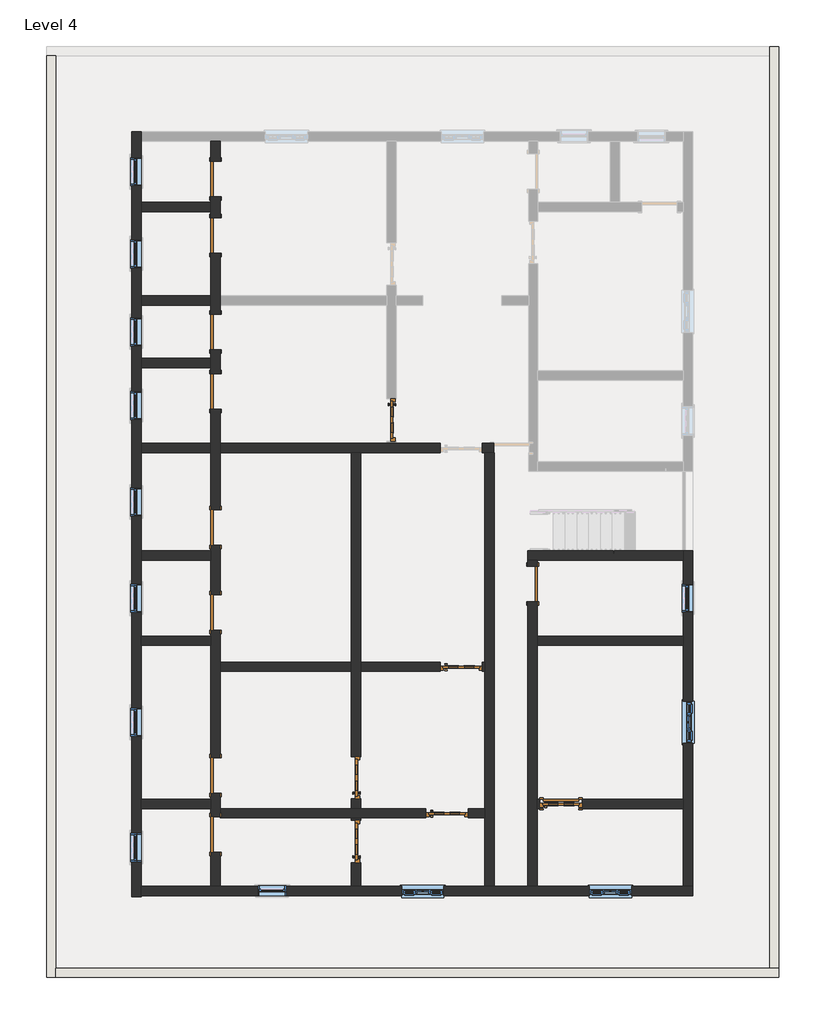
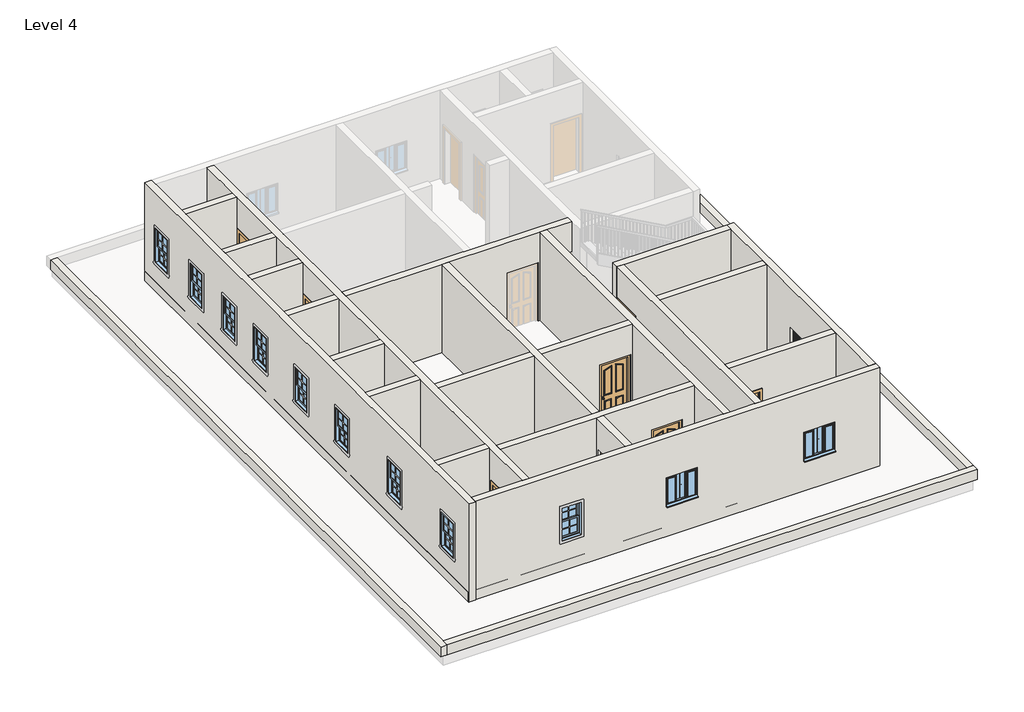
# One storey, part 1 of 3: 22 walls, 16 doors, 13 windows.
"""IFC4 building model written with IfcOpenShell, lengths in millimetres."""

from ifc_helpers import new_model, si_unit, frame, origin, place, context, project, spatial, polyline, outline, extrude, faceted_brep, transform, mapped, element, save
from components import doors_extsgl_12_910x2110mm_9a09825e, doors_extsgl_12_910x2110mm_ece77ece, door_fadea3f2, door_53b1b562, window_679d2811, windows_tpl_w_glazing_cross_bars_910x910mm_4aa0f884

model = new_model("IFC4")

# Units and contexts
model_context = context("Model", 3, world=origin())
ifc_project = project(units=[si_unit("LENGTHUNIT", "METRE", prefix="MILLI")], contexts=[model_context])

# Site, building, storey
site = spatial("IfcSite", under=ifc_project)
building = spatial("IfcBuilding", under=site)
storey = spatial("IfcBuildingStorey", under=building, Name="Level 4", Elevation=9144.0)

# Doors
placement = place(None, origin())
doors_extsgl_12_910x2110mm_shape = doors_extsgl_12_910x2110mm_9a09825e(model_context)
element("IfcDoor", 1, ObjectType="Doors_ExtSgl_12 : 910x2110mm", at=placement, inside=storey, context=model_context, shape_type="MappedRepresentation", body=[
    mapped(doors_extsgl_12_910x2110mm_shape, transform((-4887.6876145, 1213.3404944, 9144.0), x_axis=(0.0, -1.0, 0.0), y_axis=(1.0, 0.0, 0.0), z_axis=(0.0, 0.0, 1.0))),
])
doors_extsgl_12_910x2110mm_2_shape = doors_extsgl_12_910x2110mm_ece77ece(model_context)
element("IfcDoor", 2, ObjectType="Doors_ExtSgl_12 : 910x2110mm", at=placement, inside=storey, context=model_context, shape_type="MappedRepresentation", body=[
    mapped(doors_extsgl_12_910x2110mm_2_shape, transform((-5649.6876145, -6482.8595056, 9144.0), x_axis=(0.0, 1.0, 0.0), y_axis=(-1.0, 0.0, 0.0), z_axis=(0.0, 0.0, 1.0))),
])
element("IfcDoor", 3, ObjectType="Doors_ExtSgl_12 : 910x2110mm", at=placement, inside=storey, context=model_context, shape_type="MappedRepresentation", body=[
    mapped(doors_extsgl_12_910x2110mm_2_shape, transform((-1242.7876145, -7041.6595056, 9144.0), x_axis=(1.0, 0.0, 0.0), y_axis=(0.0, 1.0, 0.0), z_axis=(0.0, 0.0, 1.0))),
])
element("IfcDoor", 4, ObjectType="Doors_ExtSgl_12 : 910x2110mm", at=placement, inside=storey, context=model_context, shape_type="MappedRepresentation", body=[
    mapped(doors_extsgl_12_910x2110mm_2_shape, transform((-5649.6876145, -7854.4595056, 9144.0), x_axis=(0.0, 1.0, 0.0), y_axis=(-1.0, 0.0, 0.0), z_axis=(0.0, 0.0, 1.0))),
])
element("IfcDoor", 5, ObjectType="Doors_ExtSgl_12 : 910x2110mm", at=placement, inside=storey, context=model_context, shape_type="MappedRepresentation", body=[
    mapped(doors_extsgl_12_910x2110mm_2_shape, transform((-3693.8876145, -7244.8595056, 9144.0), x_axis=(1.0, 0.0, 0.0), y_axis=(0.0, 1.0, 0.0), z_axis=(0.0, 0.0, 1.0))),
])
element("IfcDoor", 6, ObjectType="Doors_ExtSgl_12 : 910x2110mm", at=placement, inside=storey, context=model_context, shape_type="MappedRepresentation", body=[
    mapped(doors_extsgl_12_910x2110mm_2_shape, transform((-3389.0876145, -4095.2595056, 9144.0), x_axis=(1.0, 0.0, 0.0), y_axis=(0.0, 1.0, 0.0), z_axis=(0.0, 0.0, 1.0))),
])
door_shape = door_fadea3f2(model_context)
element("IfcDoor", 7, ObjectType="Single-Flush : 30\" x 80\"", at=placement, inside=storey, context=model_context, shape_type="MappedRepresentation", body=[
    mapped(door_shape, transform((-8672.2876145, 5175.7404944, 9144.0), x_axis=(0.0, 1.0, 0.0), y_axis=(-1.0, 0.0, 0.0), z_axis=(0.0, 0.0, 1.0))),
])
element("IfcDoor", 8, ObjectType="Single-Flush : 30\" x 80\"", at=placement, inside=storey, context=model_context, shape_type="MappedRepresentation", body=[
    mapped(door_shape, transform((-8672.2876145, -7702.0595056, 9144.0), x_axis=(0.0, 1.0, 0.0), y_axis=(-1.0, 0.0, 0.0), z_axis=(0.0, 0.0, 1.0))),
])
element("IfcDoor", 9, ObjectType="Single-Flush : 30\" x 80\"", at=placement, inside=storey, context=model_context, shape_type="MappedRepresentation", body=[
    mapped(door_shape, transform((-1852.3876145, -2317.2595056, 9144.0), x_axis=(0.0, -1.0, 0.0), y_axis=(1.0, 0.0, 0.0), z_axis=(0.0, 0.0, 1.0))),
])
element("IfcDoor", 10, ObjectType="Single-Flush : 30\" x 80\"", at=placement, inside=storey, context=model_context, shape_type="MappedRepresentation", body=[
    mapped(door_shape, transform((-1242.7876145, -7041.6595056, 9144.0), x_axis=(1.0, 0.0, 0.0), y_axis=(0.0, 1.0, 0.0), z_axis=(0.0, 0.0, 1.0))),
])
door_2_shape = door_53b1b562(model_context)
element("IfcDoor", 11, ObjectType="Single-Flush : 30\" x 80\"", at=placement, inside=storey, context=model_context, shape_type="MappedRepresentation", body=[
    mapped(door_2_shape, transform((-8672.2876145, 6394.9404944, 9144.0), x_axis=(0.0, -1.0, 0.0), y_axis=(1.0, 0.0, 0.0), z_axis=(0.0, 0.0, 1.0))),
])
element("IfcDoor", 12, ObjectType="Single-Flush : 30\" x 80\"", at=placement, inside=storey, context=model_context, shape_type="MappedRepresentation", body=[
    mapped(door_2_shape, transform((-8672.2876145, 3105.6404944, 9144.0), x_axis=(0.0, -1.0, 0.0), y_axis=(1.0, 0.0, 0.0), z_axis=(0.0, 0.0, 1.0))),
])
element("IfcDoor", 13, ObjectType="Single-Flush : 30\" x 80\"", at=placement, inside=storey, context=model_context, shape_type="MappedRepresentation", body=[
    mapped(door_2_shape, transform((-8672.2876145, 1822.9404944, 9144.0), x_axis=(0.0, -1.0, 0.0), y_axis=(1.0, 0.0, 0.0), z_axis=(0.0, 0.0, 1.0))),
])
element("IfcDoor", 14, ObjectType="Single-Flush : 30\" x 80\"", at=placement, inside=storey, context=model_context, shape_type="MappedRepresentation", body=[
    mapped(door_2_shape, transform((-8672.2876145, -1098.0595056, 9144.0), x_axis=(0.0, -1.0, 0.0), y_axis=(1.0, 0.0, 0.0), z_axis=(0.0, 0.0, 1.0))),
])
element("IfcDoor", 15, ObjectType="Single-Flush : 30\" x 80\"", at=placement, inside=storey, context=model_context, shape_type="MappedRepresentation", body=[
    mapped(door_2_shape, transform((-8672.2876145, -2926.8595056, 9144.0), x_axis=(0.0, -1.0, 0.0), y_axis=(1.0, 0.0, 0.0), z_axis=(0.0, 0.0, 1.0))),
])
element("IfcDoor", 16, ObjectType="Single-Flush : 30\" x 80\"", at=placement, inside=storey, context=model_context, shape_type="MappedRepresentation", body=[
    mapped(door_2_shape, transform((-8672.2876145, -6432.0595056, 9144.0), x_axis=(0.0, -1.0, 0.0), y_axis=(1.0, 0.0, 0.0), z_axis=(0.0, 0.0, 1.0))),
])

# Walls
element("IfcWall", 17, ObjectType="4.5\"", at=placement, inside=storey, context=model_context, shape_type="Brep", body=[
    faceted_brep([(-8773.8876145, -6813.0595056, 9144.0), (-8773.8876145, -6940.0595056, 9144.0), (-8773.8876145, -7143.2595056, 9144.0), (-8773.8876145, -7321.0595056, 9144.0), (-8773.8876145, -7321.0595056, 11176.0), (-8773.8876145, -8083.0595056, 11176.0), (-8773.8876145, -8083.0595056, 9144.0), (-8773.8876145, -8819.6595056, 9144.0), (-8773.8876145, -8819.6595056, 12192.0), (-8773.8876145, -7143.2595056, 12192.0), (-8773.8876145, -6940.0595056, 12192.0), (-8773.8876145, -3638.0595056, 12192.0), (-8773.8876145, -3434.8595056, 12192.0), (-8773.8876145, -1809.2595056, 12192.0), (-8773.8876145, -1606.0595056, 12192.0), (-8773.8876145, 502.1404944, 12192.0), (-8773.8876145, 705.3404944, 12192.0), (-8773.8876145, 2330.9404944, 12192.0), (-8773.8876145, 2534.1404944, 12192.0), (-8773.8876145, 3677.1404944, 12192.0), (-8773.8876145, 3880.3404944, 12192.0), (-8773.8876145, 5683.7404944, 12192.0), (-8773.8876145, 5886.9404944, 12192.0), (-8773.8876145, 7207.7404944, 12192.0), (-8773.8876145, 7207.7404944, 9144.0), (-8773.8876145, 6775.9404944, 9144.0), (-8773.8876145, 6775.9404944, 11176.0), (-8773.8876145, 6013.9404944, 11176.0), (-8773.8876145, 6013.9404944, 9144.0), (-8773.8876145, 5886.9404944, 9144.0), (-8773.8876145, 5683.7404944, 9144.0), (-8773.8876145, 5556.7404944, 9144.0), (-8773.8876145, 5556.7404944, 11176.0), (-8773.8876145, 4794.7404944, 11176.0), (-8773.8876145, 4794.7404944, 9144.0), (-8773.8876145, 3880.3404944, 9144.0), (-8773.8876145, 3677.1404944, 9144.0), (-8773.8876145, 3486.6404944, 9144.0), (-8773.8876145, 3486.6404944, 11176.0), (-8773.8876145, 2724.6404944, 11176.0), (-8773.8876145, 2724.6404944, 9144.0), (-8773.8876145, 2534.1404944, 9144.0), (-8773.8876145, 2330.9404944, 9144.0), (-8773.8876145, 2203.9404944, 9144.0), (-8773.8876145, 2203.9404944, 11176.0), (-8773.8876145, 1441.9404944, 11176.0), (-8773.8876145, 1441.9404944, 9144.0), (-8773.8876145, 705.3404944, 9144.0), (-8773.8876145, 502.1404944, 9144.0), (-8773.8876145, -717.0595056, 9144.0), (-8773.8876145, -717.0595056, 11176.0), (-8773.8876145, -1479.0595056, 11176.0), (-8773.8876145, -1479.0595056, 9144.0), (-8773.8876145, -1606.0595056, 9144.0), (-8773.8876145, -1809.2595056, 9144.0), (-8773.8876145, -2545.8595056, 9144.0), (-8773.8876145, -2545.8595056, 11176.0), (-8773.8876145, -3307.8595056, 11176.0), (-8773.8876145, -3307.8595056, 9144.0), (-8773.8876145, -3434.8595056, 9144.0), (-8773.8876145, -3638.0595056, 9144.0), (-8773.8876145, -6051.0595056, 9144.0), (-8773.8876145, -6051.0595056, 11176.0), (-8773.8876145, -6813.0595056, 11176.0), (-8570.6876145, -7321.0595056, 11176.0), (-8570.6876145, -7321.0595056, 9144.0), (-8570.6876145, -7143.2595056, 9144.0), (-8570.6876145, -6813.0595056, 9144.0), (-8570.6876145, -6813.0595056, 11176.0), (-8570.6876145, -6051.0595056, 11176.0), (-8570.6876145, -6051.0595056, 9144.0), (-8570.6876145, -4196.8595056, 9144.0), (-8570.6876145, -3993.6595056, 9144.0), (-8570.6876145, -3307.8595056, 9144.0), (-8570.6876145, -3307.8595056, 11176.0), (-8570.6876145, -2545.8595056, 11176.0), (-8570.6876145, -2545.8595056, 9144.0), (-8570.6876145, -1479.0595056, 9144.0), (-8570.6876145, -1479.0595056, 11176.0), (-8570.6876145, -717.0595056, 11176.0), (-8570.6876145, -717.0595056, 9144.0), (-8570.6876145, 502.1404944, 9144.0), (-8570.6876145, 705.3404944, 9144.0), (-8570.6876145, 1441.9404944, 9144.0), (-8570.6876145, 1441.9404944, 11176.0), (-8570.6876145, 2203.9404944, 11176.0), (-8570.6876145, 2203.9404944, 9144.0), (-8570.6876145, 2724.6404944, 9144.0), (-8570.6876145, 2724.6404944, 11176.0), (-8570.6876145, 3486.6404944, 11176.0), (-8570.6876145, 3486.6404944, 9144.0), (-8570.6876145, 3677.1404944, 9144.0), (-8570.6876145, 3880.3404944, 9144.0), (-8570.6876145, 4794.7404944, 9144.0), (-8570.6876145, 4794.7404944, 11176.0), (-8570.6876145, 5556.7404944, 11176.0), (-8570.6876145, 5556.7404944, 9144.0), (-8570.6876145, 6013.9404944, 9144.0), (-8570.6876145, 6013.9404944, 11176.0), (-8570.6876145, 6775.9404944, 11176.0), (-8570.6876145, 6775.9404944, 9144.0), (-8570.6876145, 7207.7404944, 9144.0), (-8570.6876145, 7207.7404944, 12192.0), (-8570.6876145, 3880.3404944, 12192.0), (-8570.6876145, 3677.1404944, 12192.0), (-8570.6876145, 705.3404944, 12192.0), (-8570.6876145, 502.1404944, 12192.0), (-8570.6876145, -3993.6595056, 12192.0), (-8570.6876145, -4196.8595056, 12192.0), (-8570.6876145, -7143.2595056, 12192.0), (-8570.6876145, -7346.4595056, 12192.0), (-8570.6876145, -8819.6595056, 12192.0), (-8570.6876145, -8819.6595056, 9144.0), (-8570.6876145, -8083.0595056, 9144.0), (-8570.6876145, -8083.0595056, 11176.0)], [[[0, 1, 2, 3, 4, 5, 6, 7, 8, 9, 10, 11, 12, 13, 14, 15, 16, 17, 18, 19, 20, 21, 22, 23, 24, 25, 26, 27, 28, 29, 30, 31, 32, 33, 34, 35, 36, 37, 38, 39, 40, 41, 42, 43, 44, 45, 46, 47, 48, 49, 50, 51, 52, 53, 54, 55, 56, 57, 58, 59, 60, 61, 62, 63]], [[64, 65, 66, 67, 68, 69, 70, 71, 72, 73, 74, 75, 76, 77, 78, 79, 80, 81, 82, 83, 84, 85, 86, 87, 88, 89, 90, 91, 92, 93, 94, 95, 96, 97, 98, 99, 100, 101, 102, 103, 104, 105, 106, 107, 108, 109, 110, 111, 112, 113, 114]], [[25, 24, 101, 100]], [[97, 96, 31, 30, 29, 28]], [[37, 36, 35, 34, 93, 92, 91, 90]], [[43, 42, 41, 40, 87, 86]], [[49, 48, 47, 46, 83, 82, 81, 80]], [[55, 54, 53, 52, 77, 76]], [[61, 60, 59, 58, 73, 72, 71, 70]], [[113, 112, 7, 6]], [[67, 66, 65, 3, 2, 1, 0]], [[23, 22, 21, 20, 19, 18, 17, 16, 15, 14, 13, 12, 11, 10, 9, 8, 111, 110, 109, 108, 107, 106, 105, 104, 103, 102]], [[8, 7, 112, 111]], [[24, 23, 102, 101]], [[98, 97, 28, 27]], [[99, 98, 27, 26]], [[100, 99, 26, 25]], [[32, 31, 96, 95]], [[33, 32, 95, 94]], [[34, 33, 94, 93]], [[88, 87, 40, 39]], [[89, 88, 39, 38]], [[90, 89, 38, 37]], [[84, 83, 46, 45]], [[85, 84, 45, 44]], [[86, 85, 44, 43]], [[78, 77, 52, 51]], [[79, 78, 51, 50]], [[80, 79, 50, 49]], [[74, 73, 58, 57]], [[75, 74, 57, 56]], [[76, 75, 56, 55]], [[68, 67, 0, 63]], [[69, 68, 63, 62]], [[70, 69, 62, 61]], [[4, 3, 65, 64]], [[5, 4, 64, 114]], [[6, 5, 114, 113]]]),
])
element("IfcWall", 18, ObjectType="4.5\"", at=placement, inside=storey, context=model_context, shape_type="SweptSolid", body=[
    extrude(outline(polyline([(-8773.8876145, 5683.7404944), (-10272.4876145, 5683.7404944), (-10272.4876145, 5886.9404944), (-8773.8876145, 5886.9404944), (-8773.8876145, 5683.7404944)])), frame((0.0, 0.0, 9144.0), z_axis=(0.0, 0.0, 1.0), x_axis=(1.0, 0.0, 0.0)), (0.0, 0.0, 1.0), 3048.0),
])
element("IfcWall", 19, ObjectType="4.5\"", at=placement, inside=storey, context=model_context, shape_type="SweptSolid", body=[
    extrude(outline(polyline([(-8773.8876145, 3677.1404944), (-10272.4876145, 3677.1404944), (-10272.4876145, 3880.3404944), (-8773.8876145, 3880.3404944), (-8773.8876145, 3677.1404944)])), frame((0.0, 0.0, 9144.0), z_axis=(0.0, 0.0, 1.0), x_axis=(1.0, 0.0, 0.0)), (0.0, 0.0, 1.0), 3048.0),
])
element("IfcWall", 20, ObjectType="4.5\"", at=placement, inside=storey, context=model_context, shape_type="SweptSolid", body=[
    extrude(outline(polyline([(-8773.8876145, 2330.9404944), (-10272.4876145, 2330.9404944), (-10272.4876145, 2534.1404944), (-8773.8876145, 2534.1404944), (-8773.8876145, 2330.9404944)])), frame((0.0, 0.0, 9144.0), z_axis=(0.0, 0.0, 1.0), x_axis=(1.0, 0.0, 0.0)), (0.0, 0.0, 1.0), 3048.0),
])
element("IfcWall", 21, ObjectType="4.5\"", at=placement, inside=storey, context=model_context, shape_type="Brep", body=[
    faceted_brep([(-10272.4876145, 502.1404944, 12192.0), (-10272.4876145, 502.1404944, 9144.0), (-8773.8876145, 502.1404944, 9144.0), (-8773.8876145, 502.1404944, 12192.0), (-10272.4876145, 705.3404944, 9144.0), (-10272.4876145, 705.3404944, 12192.0), (-8773.8876145, 705.3404944, 12192.0), (-8773.8876145, 705.3404944, 9144.0)], [[[0, 1, 2, 3]], [[4, 5, 6, 7]], [[1, 4, 7, 2]], [[5, 0, 3, 6]], [[1, 0, 5, 4]], [[3, 2, 7, 6]]]),
    faceted_brep([(-1941.2876145, 502.1404944, 11176.0), (-1941.2876145, 502.1404944, 12192.0), (-2677.8876145, 502.1404944, 12192.0), (-2881.0876145, 502.1404944, 12192.0), (-5548.0876145, 502.1404944, 12192.0), (-5751.2876145, 502.1404944, 12192.0), (-8570.6876145, 502.1404944, 12192.0), (-8570.6876145, 502.1404944, 9144.0), (-5751.2876145, 502.1404944, 9144.0), (-5548.0876145, 502.1404944, 9144.0), (-3844.0876145, 502.1404944, 9144.0), (-3844.0876145, 502.1404944, 11254.0), (-2934.0876145, 502.1404944, 11254.0), (-2934.0876145, 502.1404944, 9144.0), (-2881.0876145, 502.1404944, 9144.0), (-2690.5876145, 502.1404944, 9144.0), (-2690.5876145, 502.1404944, 11176.0), (-1941.2876145, 705.3404944, 12192.0), (-1941.2876145, 705.3404944, 11176.0), (-2690.5876145, 705.3404944, 11176.0), (-2690.5876145, 705.3404944, 9144.0), (-2934.0876145, 705.3404944, 9144.0), (-2934.0876145, 705.3404944, 11254.0), (-3844.0876145, 705.3404944, 11254.0), (-3844.0876145, 705.3404944, 9144.0), (-4786.0876145, 705.3404944, 9144.0), (-4989.2876145, 705.3404944, 9144.0), (-8570.6876145, 705.3404944, 9144.0), (-8570.6876145, 705.3404944, 12192.0), (-4989.2876145, 705.3404944, 12192.0), (-4786.0876145, 705.3404944, 12192.0)], [[[0, 1, 2, 3, 4, 5, 6, 7, 8, 9, 10, 11, 12, 13, 14, 15, 16]], [[17, 18, 19, 20, 21, 22, 23, 24, 25, 26, 27, 28, 29, 30]], [[20, 15, 14, 13, 21]], [[24, 10, 9, 8, 7, 27, 26, 25]], [[1, 17, 30, 29, 28, 6, 5, 4, 3, 2]], [[7, 6, 28, 27]], [[17, 1, 0, 18]], [[16, 19, 18, 0]], [[19, 16, 15, 20]], [[24, 23, 11, 10]], [[22, 21, 13, 12]], [[23, 22, 12, 11]]]),
])
element("IfcWall", 22, ObjectType="4.5\"", at=placement, inside=storey, context=model_context, shape_type="SweptSolid", body=[
    extrude(outline(polyline([(-8773.8876145, -1809.2595056), (-10272.4876145, -1809.2595056), (-10272.4876145, -1606.0595056), (-8773.8876145, -1606.0595056), (-8773.8876145, -1809.2595056)])), frame((0.0, 0.0, 9144.0), z_axis=(0.0, 0.0, 1.0), x_axis=(1.0, 0.0, 0.0)), (0.0, 0.0, 1.0), 3048.0),
])
element("IfcWall", 23, ObjectType="4.5\"", at=placement, inside=storey, context=model_context, shape_type="SweptSolid", body=[
    extrude(outline(polyline([(-8773.8876145, -3638.0595056), (-10272.4876145, -3638.0595056), (-10272.4876145, -3434.8595056), (-8773.8876145, -3434.8595056), (-8773.8876145, -3638.0595056)])), frame((0.0, 0.0, 9144.0), z_axis=(0.0, 0.0, 1.0), x_axis=(1.0, 0.0, 0.0)), (0.0, 0.0, 1.0), 3048.0),
])
element("IfcWall", 24, ObjectType="4.5\"", at=placement, inside=storey, context=model_context, shape_type="SweptSolid", body=[
    extrude(outline(polyline([(-8773.8876145, -7143.2595056), (-10272.4876145, -7143.2595056), (-10272.4876145, -6940.0595056), (-8773.8876145, -6940.0595056), (-8773.8876145, -7143.2595056)])), frame((0.0, 0.0, 9144.0), z_axis=(0.0, 0.0, 1.0), x_axis=(1.0, 0.0, 0.0)), (0.0, 0.0, 1.0), 3048.0),
])
element("IfcWall", 25, ObjectType="4.5\"", at=placement, inside=storey, context=model_context, shape_type="Brep", body=[
    faceted_brep([(-3238.8876145, -7346.4595056, 11254.0), (-3238.8876145, -7346.4595056, 9144.0), (-2881.0876145, -7346.4595056, 9144.0), (-2881.0876145, -7346.4595056, 12192.0), (-5548.0876145, -7346.4595056, 12192.0), (-5751.2876145, -7346.4595056, 12192.0), (-8570.6876145, -7346.4595056, 12192.0), (-8570.6876145, -7346.4595056, 9144.0), (-5751.2876145, -7346.4595056, 9144.0), (-5548.0876145, -7346.4595056, 9144.0), (-4148.8876145, -7346.4595056, 9144.0), (-4148.8876145, -7346.4595056, 11254.0), (-2881.0876145, -7143.2595056, 9144.0), (-3238.8876145, -7143.2595056, 9144.0), (-3238.8876145, -7143.2595056, 11254.0), (-4148.8876145, -7143.2595056, 11254.0), (-4148.8876145, -7143.2595056, 9144.0), (-5548.0876145, -7143.2595056, 9144.0), (-5751.2876145, -7143.2595056, 9144.0), (-8570.6876145, -7143.2595056, 9144.0), (-8570.6876145, -7143.2595056, 12192.0), (-5751.2876145, -7143.2595056, 12192.0), (-5548.0876145, -7143.2595056, 12192.0), (-2881.0876145, -7143.2595056, 12192.0), (-8570.6876145, -7321.0595056, 9144.0)], [[[0, 1, 2, 3, 4, 5, 6, 7, 8, 9, 10, 11]], [[12, 13, 14, 15, 16, 17, 18, 19, 20, 21, 22, 23]], [[2, 1, 13, 12]], [[10, 9, 8, 7, 24, 19, 18, 17, 16]], [[6, 5, 4, 3, 23, 22, 21, 20]], [[7, 6, 20, 19, 24]], [[3, 2, 12, 23]], [[16, 15, 11, 10]], [[14, 13, 1, 0]], [[15, 14, 0, 11]]]),
])
element("IfcWall", 26, ObjectType="4.5\"", at=placement, inside=storey, context=model_context, shape_type="Brep", body=[
    faceted_brep([(-5751.2876145, -8819.6595056, 9144.0), (-5751.2876145, -8819.6595056, 12192.0), (-5751.2876145, -7346.4595056, 12192.0), (-5751.2876145, -7346.4595056, 9144.0), (-5751.2876145, -7399.4595056, 9144.0), (-5751.2876145, -7399.4595056, 11254.0), (-5751.2876145, -8309.4595056, 11254.0), (-5751.2876145, -8309.4595056, 9144.0), (-5548.0876145, -8819.6595056, 12192.0), (-5548.0876145, -8819.6595056, 9144.0), (-5548.0876145, -8309.4595056, 9144.0), (-5548.0876145, -8309.4595056, 11254.0), (-5548.0876145, -7399.4595056, 11254.0), (-5548.0876145, -7399.4595056, 9144.0), (-5548.0876145, -7346.4595056, 9144.0), (-5548.0876145, -7346.4595056, 12192.0)], [[[0, 1, 2, 3, 4, 5, 6, 7]], [[8, 9, 10, 11, 12, 13, 14, 15]], [[9, 0, 7, 10]], [[13, 4, 3, 14]], [[1, 8, 15, 2]], [[1, 0, 9, 8]], [[3, 2, 15, 14]], [[7, 6, 11, 10]], [[5, 4, 13, 12]], [[6, 5, 12, 11]]]),
    faceted_brep([(-5751.2876145, 502.1404944, 12192.0), (-5751.2876145, 502.1404944, 9144.0), (-5751.2876145, -3993.6595056, 9144.0), (-5751.2876145, -4196.8595056, 9144.0), (-5751.2876145, -6027.8595056, 9144.0), (-5751.2876145, -6027.8595056, 11254.0), (-5751.2876145, -6937.8595056, 11254.0), (-5751.2876145, -6937.8595056, 9144.0), (-5751.2876145, -7143.2595056, 9144.0), (-5751.2876145, -7143.2595056, 12192.0), (-5751.2876145, -4196.8595056, 12192.0), (-5751.2876145, -3993.6595056, 12192.0), (-5548.0876145, 502.1404944, 9144.0), (-5548.0876145, 502.1404944, 12192.0), (-5548.0876145, -3993.6595056, 12192.0), (-5548.0876145, -4196.8595056, 12192.0), (-5548.0876145, -7143.2595056, 12192.0), (-5548.0876145, -7143.2595056, 9144.0), (-5548.0876145, -6937.8595056, 9144.0), (-5548.0876145, -6937.8595056, 11254.0), (-5548.0876145, -6027.8595056, 11254.0), (-5548.0876145, -6027.8595056, 9144.0), (-5548.0876145, -4196.8595056, 9144.0), (-5548.0876145, -3993.6595056, 9144.0)], [[[0, 1, 2, 3, 4, 5, 6, 7, 8, 9, 10, 11]], [[12, 13, 14, 15, 16, 17, 18, 19, 20, 21, 22, 23]], [[1, 12, 23, 22, 21, 4, 3, 2]], [[7, 18, 17, 8]], [[13, 0, 11, 10, 9, 16, 15, 14]], [[1, 0, 13, 12]], [[9, 8, 17, 16]], [[7, 6, 19, 18]], [[5, 4, 21, 20]], [[6, 5, 20, 19]]]),
])
element("IfcWall", 27, ObjectType="4.5\"", at=placement, inside=storey, context=model_context, shape_type="SweptSolid", body=[
    extrude(outline(polyline([(-8570.6876145, -4196.8595056), (-8570.6876145, -3993.6595056), (-5751.2876145, -3993.6595056), (-5751.2876145, -4196.8595056), (-8570.6876145, -4196.8595056)])), frame((0.0, 0.0, 9144.0), z_axis=(0.0, 0.0, 1.0), x_axis=(1.0, 0.0, 0.0)), (0.0, 0.0, 1.0), 3048.0),
    extrude(outline(polyline([(9144.0, -2881.0876145), (12192.0, -2881.0876145), (12192.0, -5548.0876145), (9144.0, -5548.0876145), (9144.0, -3844.0876145), (11254.0, -3844.0876145), (11254.0, -2934.0876145), (9144.0, -2934.0876145), (9144.0, -2881.0876145)])), frame((0.0, -4196.8595056, 0.0), z_axis=(0.0, 1.0, 0.0), x_axis=(0.0, 0.0, 1.0)), (0.0, 0.0, 1.0), 203.2),
])
element("IfcWall", 28, ObjectType="4.5\"", at=placement, inside=storey, context=model_context, shape_type="Brep", body=[
    faceted_brep([(-2881.0876145, 502.1404944, 9144.0), (-2881.0876145, -3993.6595056, 9144.0), (-2881.0876145, -4196.8595056, 9144.0), (-2881.0876145, -7143.2595056, 9144.0), (-2881.0876145, -7346.4595056, 9144.0), (-2881.0876145, -8819.6595056, 9144.0), (-2881.0876145, -8819.6595056, 12192.0), (-2881.0876145, -7346.4595056, 12192.0), (-2881.0876145, -7143.2595056, 12192.0), (-2881.0876145, -4196.8595056, 12192.0), (-2881.0876145, -3993.6595056, 12192.0), (-2881.0876145, 502.1404944, 12192.0), (-2677.8876145, 502.1404944, 9144.0), (-2677.8876145, 502.1404944, 12192.0), (-2677.8876145, -8819.6595056, 12192.0), (-2677.8876145, -8819.6595056, 9144.0), (-2690.5876145, 502.1404944, 9144.0)], [[[0, 1, 2, 3, 4, 5, 6, 7, 8, 9, 10, 11]], [[12, 13, 14, 15]], [[5, 4, 3, 2, 1, 0, 16, 12, 15]], [[11, 10, 9, 8, 7, 6, 14, 13]], [[6, 5, 15, 14]], [[0, 11, 13, 12, 16]]]),
])
element("IfcWall", 29, ObjectType="4.5\"", at=placement, inside=storey, context=model_context, shape_type="Brep", body=[
    faceted_brep([(1386.1123855, -1606.0595056, 9144.0), (-1953.9876145, -1606.0595056, 9144.0), (-1953.9876145, -1606.0595056, 12192.0), (1386.1123855, -1606.0595056, 12192.0), (1386.1123855, -1809.2595056, 9144.0), (1386.1123855, -1809.2595056, 12192.0), (-1750.7876145, -1809.2595056, 12192.0), (-1953.9876145, -1809.2595056, 12192.0), (-1953.9876145, -1809.2595056, 9144.0), (-1750.7876145, -1809.2595056, 9144.0)], [[[0, 1, 2, 3]], [[4, 5, 6, 7, 8, 9]], [[1, 0, 4, 9, 8]], [[3, 2, 7, 6, 5]], [[0, 3, 5, 4]], [[2, 1, 8, 7]]]),
])
element("IfcWall", 30, ObjectType="4.5\"", at=placement, inside=storey, context=model_context, shape_type="Brep", body=[
    faceted_brep([(-1953.9876145, -2698.2595056, 11176.0), (-1953.9876145, -2698.2595056, 9144.0), (-1953.9876145, -8819.6595056, 9144.0), (-1953.9876145, -8819.6595056, 12192.0), (-1953.9876145, -1809.2595056, 12192.0), (-1953.9876145, -1809.2595056, 9144.0), (-1953.9876145, -1936.2595056, 9144.0), (-1953.9876145, -1936.2595056, 11176.0), (-1750.7876145, -8819.6595056, 9144.0), (-1750.7876145, -7143.2595056, 9144.0), (-1750.7876145, -6940.0595056, 9144.0), (-1750.7876145, -3638.0595056, 9144.0), (-1750.7876145, -3434.8595056, 9144.0), (-1750.7876145, -2698.2595056, 9144.0), (-1750.7876145, -2698.2595056, 11176.0), (-1750.7876145, -1936.2595056, 11176.0), (-1750.7876145, -1936.2595056, 9144.0), (-1750.7876145, -1809.2595056, 9144.0), (-1750.7876145, -1809.2595056, 12192.0), (-1750.7876145, -3434.8595056, 12192.0), (-1750.7876145, -3638.0595056, 12192.0), (-1750.7876145, -6940.0595056, 12192.0), (-1750.7876145, -7143.2595056, 12192.0), (-1750.7876145, -8819.6595056, 12192.0)], [[[0, 1, 2, 3, 4, 5, 6, 7]], [[8, 9, 10, 11, 12, 13, 14, 15, 16, 17, 18, 19, 20, 21, 22, 23]], [[6, 5, 17, 16]], [[2, 1, 13, 12, 11, 10, 9, 8]], [[4, 3, 23, 22, 21, 20, 19, 18]], [[5, 4, 18, 17]], [[3, 2, 8, 23]], [[14, 13, 1, 0]], [[15, 14, 0, 7]], [[16, 15, 7, 6]]]),
])
element("IfcWall", 31, ObjectType="4.5\"", at=placement, inside=storey, context=model_context, shape_type="SweptSolid", body=[
    extrude(outline(polyline([(12192.0, 1386.1123855), (12192.0, -1750.7876145), (9144.0, -1750.7876145), (9144.0, -1697.7876145), (11254.0, -1697.7876145), (11254.0, -787.7876145), (9144.0, -787.7876145), (9144.0, 1386.1123855), (12192.0, 1386.1123855)])), frame((0.0, -7143.2595056, 0.0), z_axis=(0.0, 1.0, 0.0), x_axis=(0.0, 0.0, 1.0)), (0.0, 0.0, 1.0), 203.2),
])
element("IfcWall", 32, ObjectType="4.5\"", at=placement, inside=storey, context=model_context, shape_type="SweptSolid", body=[
    extrude(outline(polyline([(1386.1123855, -3638.0595056), (-1750.7876145, -3638.0595056), (-1750.7876145, -3434.8595056), (1386.1123855, -3434.8595056), (1386.1123855, -3638.0595056)])), frame((0.0, 0.0, 9144.0), z_axis=(0.0, 0.0, 1.0), x_axis=(1.0, 0.0, 0.0)), (0.0, 0.0, 1.0), 3048.0),
])
element("IfcWall", 33, ObjectType="4.5\"", at=placement, inside=storey, context=model_context, shape_type="Brep", body=[
    faceted_brep([(-12101.2876145, -10775.4595056, 9144.0), (-12101.2876145, -10572.2595056, 9144.0), (-12101.2876145, 9036.5404944, 9144.0), (-12101.2876145, 9036.5404944, 9448.8), (-12101.2876145, -10572.2595056, 9448.8), (-12101.2876145, -10775.4595056, 9448.8), (-12304.4876145, -10775.4595056, 9144.0), (-12304.4876145, -10775.4595056, 9448.8), (-12304.4876145, 9036.5404944, 9448.8), (-12304.4876145, 9036.5404944, 9144.0)], [[[0, 1, 2, 3, 4, 5]], [[6, 7, 8, 9]], [[2, 1, 0, 6, 9]], [[5, 4, 3, 8, 7]], [[0, 5, 7, 6]], [[3, 2, 9, 8]]]),
])
element("IfcWall", 34, ObjectType="4.5\"", at=placement, inside=storey, context=model_context, shape_type="Brep", body=[
    faceted_brep([(3443.5123855, -10572.2595056, 9144.0), (3240.3123855, -10572.2595056, 9144.0), (-12101.2876145, -10572.2595056, 9144.0), (-12101.2876145, -10572.2595056, 9448.8), (3240.3123855, -10572.2595056, 9448.8), (3443.5123855, -10572.2595056, 9448.8), (3443.5123855, -10775.4595056, 9144.0), (3443.5123855, -10775.4595056, 9448.8), (-12101.2876145, -10775.4595056, 9448.8), (-12101.2876145, -10775.4595056, 9144.0)], [[[0, 1, 2, 3, 4, 5]], [[6, 7, 8, 9]], [[2, 1, 0, 6, 9]], [[5, 4, 3, 8, 7]], [[0, 5, 7, 6]], [[3, 2, 9, 8]]]),
])
element("IfcWall", 35, ObjectType="4.5\"", at=placement, inside=storey, context=model_context, shape_type="Brep", body=[
    faceted_brep([(3240.3123855, 9239.7404944, 9144.0), (3240.3123855, 9036.5404944, 9144.0), (3240.3123855, -10572.2595056, 9144.0), (3240.3123855, -10572.2595056, 9448.8), (3240.3123855, 9036.5404944, 9448.8), (3240.3123855, 9239.7404944, 9448.8), (3443.5123855, 9239.7404944, 9144.0), (3443.5123855, 9239.7404944, 9448.8), (3443.5123855, -10572.2595056, 9448.8), (3443.5123855, -10572.2595056, 9144.0)], [[[0, 1, 2, 3, 4, 5]], [[6, 7, 8, 9]], [[2, 1, 0, 6, 9]], [[5, 4, 3, 8, 7]], [[0, 5, 7, 6]], [[3, 2, 9, 8]]]),
])
element("IfcWall", 36, ObjectType="Generic - 9\"", at=placement, inside=storey, context=model_context, shape_type="Brep", body=[
    faceted_brep([(-10475.6876145, 7410.9404944, 9144.0), (-10475.6876145, -9035.5595056, 9144.0), (-10475.6876145, -9035.5595056, 12192.0), (-10475.6876145, 7410.9404944, 12192.0), (-10475.6876145, 6242.5404944, 11125.2), (-10475.6876145, 6242.5404944, 10058.4), (-10475.6876145, 6852.1404944, 10058.4), (-10475.6876145, 6852.1404944, 11125.2), (-10475.6876145, 4477.2404944, 11125.2), (-10475.6876145, 4477.2404944, 10058.4), (-10475.6876145, 5086.8404944, 10058.4), (-10475.6876145, 5086.8404944, 11125.2), (-10475.6876145, 2800.8404944, 11125.2), (-10475.6876145, 2800.8404944, 10058.4), (-10475.6876145, 3410.4404944, 10058.4), (-10475.6876145, 3410.4404944, 11125.2), (-10475.6876145, 1213.3404944, 11125.2), (-10475.6876145, 1213.3404944, 10058.4), (-10475.6876145, 1822.9404944, 10058.4), (-10475.6876145, 1822.9404944, 11125.2), (-10475.6876145, -856.7595056, 11125.2), (-10475.6876145, -856.7595056, 10058.4), (-10475.6876145, -247.1595056, 10058.4), (-10475.6876145, -247.1595056, 11125.2), (-10475.6876145, -2926.8595056, 11125.2), (-10475.6876145, -2926.8595056, 10058.4), (-10475.6876145, -2317.2595056, 10058.4), (-10475.6876145, -2317.2595056, 11125.2), (-10475.6876145, -5593.8595056, 11125.2), (-10475.6876145, -5593.8595056, 10058.4), (-10475.6876145, -4984.2595056, 10058.4), (-10475.6876145, -4984.2595056, 11125.2), (-10475.6876145, -8286.2595056, 11125.2), (-10475.6876145, -8286.2595056, 10058.4), (-10475.6876145, -7676.6595056, 10058.4), (-10475.6876145, -7676.6595056, 11125.2), (-10272.4876145, 7410.9404944, 9144.0), (-10272.4876145, 7410.9404944, 12192.0), (-10272.4876145, 7207.7404944, 12192.0), (-10272.4876145, 5886.9404944, 12192.0), (-10272.4876145, 5683.7404944, 12192.0), (-10272.4876145, 3880.3404944, 12192.0), (-10272.4876145, 3677.1404944, 12192.0), (-10272.4876145, 2534.1404944, 12192.0), (-10272.4876145, 2330.9404944, 12192.0), (-10272.4876145, 705.3404944, 12192.0), (-10272.4876145, 502.1404944, 12192.0), (-10272.4876145, -1606.0595056, 12192.0), (-10272.4876145, -1809.2595056, 12192.0), (-10272.4876145, -3434.8595056, 12192.0), (-10272.4876145, -3638.0595056, 12192.0), (-10272.4876145, -6940.0595056, 12192.0), (-10272.4876145, -7143.2595056, 12192.0), (-10272.4876145, -8819.6595056, 12192.0), (-10272.4876145, -9022.8595056, 12192.0), (-10272.4876145, -9035.5595056, 12192.0), (-10272.4876145, -9035.5595056, 9144.0), (-10272.4876145, -9022.8595056, 9144.0), (-10272.4876145, -8819.6595056, 9144.0), (-10272.4876145, -7143.2595056, 9144.0), (-10272.4876145, -6940.0595056, 9144.0), (-10272.4876145, -3638.0595056, 9144.0), (-10272.4876145, -3434.8595056, 9144.0), (-10272.4876145, -1809.2595056, 9144.0), (-10272.4876145, -1606.0595056, 9144.0), (-10272.4876145, 502.1404944, 9144.0), (-10272.4876145, 705.3404944, 9144.0), (-10272.4876145, 2330.9404944, 9144.0), (-10272.4876145, 2534.1404944, 9144.0), (-10272.4876145, 3677.1404944, 9144.0), (-10272.4876145, 3880.3404944, 9144.0), (-10272.4876145, 5683.7404944, 9144.0), (-10272.4876145, 5886.9404944, 9144.0), (-10272.4876145, 7207.7404944, 9144.0), (-10272.4876145, 6242.5404944, 11125.2), (-10272.4876145, 6852.1404944, 11125.2), (-10272.4876145, 6852.1404944, 10058.4), (-10272.4876145, 6242.5404944, 10058.4), (-10272.4876145, 4477.2404944, 11125.2), (-10272.4876145, 5086.8404944, 11125.2), (-10272.4876145, 5086.8404944, 10058.4), (-10272.4876145, 4477.2404944, 10058.4), (-10272.4876145, 2800.8404944, 11125.2), (-10272.4876145, 3410.4404944, 11125.2), (-10272.4876145, 3410.4404944, 10058.4), (-10272.4876145, 2800.8404944, 10058.4), (-10272.4876145, 1213.3404944, 11125.2), (-10272.4876145, 1822.9404944, 11125.2), (-10272.4876145, 1822.9404944, 10058.4), (-10272.4876145, 1213.3404944, 10058.4), (-10272.4876145, -856.7595056, 11125.2), (-10272.4876145, -247.1595056, 11125.2), (-10272.4876145, -247.1595056, 10058.4), (-10272.4876145, -856.7595056, 10058.4), (-10272.4876145, -2926.8595056, 11125.2), (-10272.4876145, -2317.2595056, 11125.2), (-10272.4876145, -2317.2595056, 10058.4), (-10272.4876145, -2926.8595056, 10058.4), (-10272.4876145, -5593.8595056, 11125.2), (-10272.4876145, -4984.2595056, 11125.2), (-10272.4876145, -4984.2595056, 10058.4), (-10272.4876145, -5593.8595056, 10058.4), (-10272.4876145, -8286.2595056, 11125.2), (-10272.4876145, -7676.6595056, 11125.2), (-10272.4876145, -7676.6595056, 10058.4), (-10272.4876145, -8286.2595056, 10058.4)], [[[0, 1, 2, 3], [4, 5, 6, 7], [8, 9, 10, 11], [12, 13, 14, 15], [16, 17, 18, 19], [20, 21, 22, 23], [24, 25, 26, 27], [28, 29, 30, 31], [32, 33, 34, 35]], [[36, 37, 38, 39, 40, 41, 42, 43, 44, 45, 46, 47, 48, 49, 50, 51, 52, 53, 54, 55, 56, 57, 58, 59, 60, 61, 62, 63, 64, 65, 66, 67, 68, 69, 70, 71, 72, 73], [74, 75, 76, 77], [78, 79, 80, 81], [82, 83, 84, 85], [86, 87, 88, 89], [90, 91, 92, 93], [94, 95, 96, 97], [98, 99, 100, 101], [102, 103, 104, 105]], [[1, 0, 36, 73, 72, 71, 70, 69, 68, 67, 66, 65, 64, 63, 62, 61, 60, 59, 58, 57, 56]], [[2, 1, 56, 55]], [[3, 2, 55, 54, 53, 52, 51, 50, 49, 48, 47, 46, 45, 44, 43, 42, 41, 40, 39, 38, 37]], [[0, 3, 37, 36]], [[5, 4, 74, 77]], [[6, 5, 77, 76]], [[7, 6, 76, 75]], [[4, 7, 75, 74]], [[9, 8, 78, 81]], [[10, 9, 81, 80]], [[11, 10, 80, 79]], [[8, 11, 79, 78]], [[13, 12, 82, 85]], [[14, 13, 85, 84]], [[15, 14, 84, 83]], [[12, 15, 83, 82]], [[17, 16, 86, 89]], [[18, 17, 89, 88]], [[19, 18, 88, 87]], [[16, 19, 87, 86]], [[21, 20, 90, 93]], [[22, 21, 93, 92]], [[23, 22, 92, 91]], [[20, 23, 91, 90]], [[25, 24, 94, 97]], [[26, 25, 97, 96]], [[27, 26, 96, 95]], [[24, 27, 95, 94]], [[29, 28, 98, 101]], [[30, 29, 101, 100]], [[31, 30, 100, 99]], [[28, 31, 99, 98]], [[33, 32, 102, 105]], [[34, 33, 105, 104]], [[35, 34, 104, 103]], [[32, 35, 103, 102]]]),
])
element("IfcWall", 37, ObjectType="Generic - 9\"", at=placement, inside=storey, context=model_context, shape_type="Brep", body=[
    faceted_brep([(-10272.4876145, -9022.8595056, 9144.0), (1589.3123855, -9022.8595056, 9144.0), (1589.3123855, -9022.8595056, 12192.0), (-10272.4876145, -9022.8595056, 12192.0), (-7757.8876145, -9022.8595056, 11125.2), (-7148.2876145, -9022.8595056, 11125.2), (-7148.2876145, -9022.8595056, 10058.4), (-7757.8876145, -9022.8595056, 10058.4), (272.6623855, -9022.8595056, 10968.4), (272.6623855, -9022.8595056, 10058.4), (-637.3376145, -9022.8595056, 10058.4), (-637.3376145, -9022.8595056, 10968.4), (-3759.5876145, -9022.8595056, 10968.4), (-3759.5876145, -9022.8595056, 10058.4), (-4669.5876145, -9022.8595056, 10058.4), (-4669.5876145, -9022.8595056, 10968.4), (-10272.4876145, -8819.6595056, 9144.0), (-10272.4876145, -8819.6595056, 12192.0), (-8773.8876145, -8819.6595056, 12192.0), (-8570.6876145, -8819.6595056, 12192.0), (-5751.2876145, -8819.6595056, 12192.0), (-5548.0876145, -8819.6595056, 12192.0), (-2881.0876145, -8819.6595056, 12192.0), (-2677.8876145, -8819.6595056, 12192.0), (-1953.9876145, -8819.6595056, 12192.0), (-1750.7876145, -8819.6595056, 12192.0), (1386.1123855, -8819.6595056, 12192.0), (1589.3123855, -8819.6595056, 12192.0), (1589.3123855, -8819.6595056, 9144.0), (1386.1123855, -8819.6595056, 9144.0), (-1750.7876145, -8819.6595056, 9144.0), (-1953.9876145, -8819.6595056, 9144.0), (-2677.8876145, -8819.6595056, 9144.0), (-2881.0876145, -8819.6595056, 9144.0), (-5548.0876145, -8819.6595056, 9144.0), (-5751.2876145, -8819.6595056, 9144.0), (-8570.6876145, -8819.6595056, 9144.0), (-8773.8876145, -8819.6595056, 9144.0), (-7757.8876145, -8819.6595056, 11125.2), (-7757.8876145, -8819.6595056, 10058.4), (-7148.2876145, -8819.6595056, 10058.4), (-7148.2876145, -8819.6595056, 11125.2), (272.6623855, -8819.6595056, 10968.4), (-637.3376145, -8819.6595056, 10968.4), (-637.3376145, -8819.6595056, 10058.4), (272.6623855, -8819.6595056, 10058.4), (-3759.5876145, -8819.6595056, 10968.4), (-4669.5876145, -8819.6595056, 10968.4), (-4669.5876145, -8819.6595056, 10058.4), (-3759.5876145, -8819.6595056, 10058.4)], [[[0, 1, 2, 3], [4, 5, 6, 7], [8, 9, 10, 11], [12, 13, 14, 15]], [[16, 17, 18, 19, 20, 21, 22, 23, 24, 25, 26, 27, 28, 29, 30, 31, 32, 33, 34, 35, 36, 37], [38, 39, 40, 41], [42, 43, 44, 45], [46, 47, 48, 49]], [[1, 0, 16, 37, 36, 35, 34, 33, 32, 31, 30, 29, 28]], [[3, 2, 27, 26, 25, 24, 23, 22, 21, 20, 19, 18, 17]], [[0, 3, 17, 16]], [[2, 1, 28, 27]], [[39, 38, 4, 7]], [[40, 39, 7, 6]], [[41, 40, 6, 5]], [[38, 41, 5, 4]], [[9, 8, 42, 45]], [[10, 9, 45, 44]], [[11, 10, 44, 43]], [[8, 11, 43, 42]], [[13, 12, 46, 49]], [[14, 13, 49, 48]], [[15, 14, 48, 47]], [[12, 15, 47, 46]]]),
])
element("IfcWall", 38, ObjectType="Generic - 9\"", at=placement, inside=storey, context=model_context, shape_type="Brep", body=[
    faceted_brep([(1589.3123855, -8819.6595056, 9144.0), (1589.3123855, -1606.0595056, 9144.0), (1589.3123855, -1606.0595056, 12192.0), (1589.3123855, -8819.6595056, 12192.0), (1589.3123855, -4834.0595056, 10968.4), (1589.3123855, -4834.0595056, 10058.4), (1589.3123855, -5744.0595056, 10058.4), (1589.3123855, -5744.0595056, 10968.4), (1589.3123855, -2926.8595056, 11125.2), (1589.3123855, -2317.2595056, 11125.2), (1589.3123855, -2317.2595056, 10058.4), (1589.3123855, -2926.8595056, 10058.4), (1386.1123855, -8819.6595056, 9144.0), (1386.1123855, -8819.6595056, 12192.0), (1386.1123855, -7143.2595056, 12192.0), (1386.1123855, -6940.0595056, 12192.0), (1386.1123855, -3638.0595056, 12192.0), (1386.1123855, -3434.8595056, 12192.0), (1386.1123855, -1809.2595056, 12192.0), (1386.1123855, -1606.0595056, 12192.0), (1386.1123855, -1606.0595056, 9144.0), (1386.1123855, -1809.2595056, 9144.0), (1386.1123855, -3434.8595056, 9144.0), (1386.1123855, -3638.0595056, 9144.0), (1386.1123855, -6940.0595056, 9144.0), (1386.1123855, -7143.2595056, 9144.0), (1386.1123855, -4834.0595056, 10968.4), (1386.1123855, -5744.0595056, 10968.4), (1386.1123855, -5744.0595056, 10058.4), (1386.1123855, -4834.0595056, 10058.4), (1386.1123855, -2926.8595056, 11125.2), (1386.1123855, -2926.8595056, 10058.4), (1386.1123855, -2317.2595056, 10058.4), (1386.1123855, -2317.2595056, 11125.2)], [[[0, 1, 2, 3], [4, 5, 6, 7], [8, 9, 10, 11]], [[12, 13, 14, 15, 16, 17, 18, 19, 20, 21, 22, 23, 24, 25], [26, 27, 28, 29], [30, 31, 32, 33]], [[1, 0, 12, 25, 24, 23, 22, 21, 20]], [[3, 2, 19, 18, 17, 16, 15, 14, 13]], [[0, 3, 13, 12]], [[2, 1, 20, 19]], [[5, 4, 26, 29]], [[6, 5, 29, 28]], [[7, 6, 28, 27]], [[4, 7, 27, 26]], [[31, 30, 8, 11]], [[32, 31, 11, 10]], [[33, 32, 10, 9]], [[30, 33, 9, 8]]]),
])

# Windows
window_shape = window_679d2811(model_context)
element("IfcWindow", 39, ObjectType="Window-Double-Hung : 24\" x 42\"", at=placement, inside=storey, context=model_context, shape_type="MappedRepresentation", body=[
    mapped(window_shape, transform((-10374.0876145, 6547.3404944, 9144.0), x_axis=(0.0, 1.0, 0.0), y_axis=(-1.0, 0.0, 0.0), z_axis=(0.0, 0.0, 1.0))),
])
element("IfcWindow", 40, ObjectType="Window-Double-Hung : 24\" x 42\"", at=placement, inside=storey, context=model_context, shape_type="MappedRepresentation", body=[
    mapped(window_shape, transform((-10374.0876145, 4782.0404944, 9144.0), x_axis=(0.0, 1.0, 0.0), y_axis=(-1.0, 0.0, 0.0), z_axis=(0.0, 0.0, 1.0))),
])
element("IfcWindow", 41, ObjectType="Window-Double-Hung : 24\" x 42\"", at=placement, inside=storey, context=model_context, shape_type="MappedRepresentation", body=[
    mapped(window_shape, transform((-10374.0876145, 3105.6404944, 9144.0), x_axis=(0.0, 1.0, 0.0), y_axis=(-1.0, 0.0, 0.0), z_axis=(0.0, 0.0, 1.0))),
])
element("IfcWindow", 42, ObjectType="Window-Double-Hung : 24\" x 42\"", at=placement, inside=storey, context=model_context, shape_type="MappedRepresentation", body=[
    mapped(window_shape, transform((-10374.0876145, 1518.1404944, 9144.0), x_axis=(0.0, 1.0, 0.0), y_axis=(-1.0, 0.0, 0.0), z_axis=(0.0, 0.0, 1.0))),
])
element("IfcWindow", 43, ObjectType="Window-Double-Hung : 24\" x 42\"", at=placement, inside=storey, context=model_context, shape_type="MappedRepresentation", body=[
    mapped(window_shape, transform((-10374.0876145, -551.9595056, 9144.0), x_axis=(0.0, 1.0, 0.0), y_axis=(-1.0, 0.0, 0.0), z_axis=(0.0, 0.0, 1.0))),
])
element("IfcWindow", 44, ObjectType="Window-Double-Hung : 24\" x 42\"", at=placement, inside=storey, context=model_context, shape_type="MappedRepresentation", body=[
    mapped(window_shape, transform((-10374.0876145, -2622.0595056, 9144.0), x_axis=(0.0, 1.0, 0.0), y_axis=(-1.0, 0.0, 0.0), z_axis=(0.0, 0.0, 1.0))),
])
element("IfcWindow", 45, ObjectType="Window-Double-Hung : 24\" x 42\"", at=placement, inside=storey, context=model_context, shape_type="MappedRepresentation", body=[
    mapped(window_shape, transform((-10374.0876145, -5289.0595056, 9144.0), x_axis=(0.0, 1.0, 0.0), y_axis=(-1.0, 0.0, 0.0), z_axis=(0.0, 0.0, 1.0))),
])
element("IfcWindow", 46, ObjectType="Window-Double-Hung : 24\" x 42\"", at=placement, inside=storey, context=model_context, shape_type="MappedRepresentation", body=[
    mapped(window_shape, transform((-10374.0876145, -7981.4595056, 9144.0), x_axis=(0.0, 1.0, 0.0), y_axis=(-1.0, 0.0, 0.0), z_axis=(0.0, 0.0, 1.0))),
])
element("IfcWindow", 47, ObjectType="Window-Double-Hung : 24\" x 42\"", at=placement, inside=storey, context=model_context, shape_type="MappedRepresentation", body=[
    mapped(window_shape, transform((-7453.0876145, -8921.2595056, 9144.0), x_axis=(1.0, 0.0, 0.0), y_axis=(0.0, 1.0, 0.0), z_axis=(0.0, 0.0, 1.0))),
])
element("IfcWindow", 48, ObjectType="Window-Double-Hung : 24\" x 42\"", at=placement, inside=storey, context=model_context, shape_type="MappedRepresentation", body=[
    mapped(window_shape, transform((1487.7123855, -2622.0595056, 9144.0), x_axis=(0.0, 1.0, 0.0), y_axis=(-1.0, 0.0, 0.0), z_axis=(0.0, 0.0, 1.0))),
])
windows_tpl_w_glazing_cross_bars_910x910mm_shape = windows_tpl_w_glazing_cross_bars_910x910mm_4aa0f884(model_context)
element("IfcWindow", 49, ObjectType="Windows_Tpl_w-Glazing_Cross-Bars : 910x910mm", at=placement, inside=storey, context=model_context, shape_type="MappedRepresentation", body=[
    mapped(windows_tpl_w_glazing_cross_bars_910x910mm_shape, transform((1479.2558177, -5715.7261723, 8858.4), x_axis=(0.0, -1.0, 0.0), y_axis=(1.0, 0.0, 0.0), z_axis=(0.0, 0.0, 1.0))),
])
element("IfcWindow", 50, ObjectType="Windows_Tpl_w-Glazing_Cross-Bars : 910x910mm", at=placement, inside=storey, context=model_context, shape_type="MappedRepresentation", body=[
    mapped(windows_tpl_w_glazing_cross_bars_910x910mm_shape, transform((-609.0042812, -8912.8029378, 8858.4), x_axis=(-1.0, 0.0, 0.0), y_axis=(0.0, -1.0, 0.0), z_axis=(0.0, 0.0, 1.0))),
])
element("IfcWindow", 51, ObjectType="Windows_Tpl_w-Glazing_Cross-Bars : 910x910mm", at=placement, inside=storey, context=model_context, shape_type="MappedRepresentation", body=[
    mapped(windows_tpl_w_glazing_cross_bars_910x910mm_shape, transform((-4641.2542812, -8912.8029378, 8858.4), x_axis=(-1.0, 0.0, 0.0), y_axis=(0.0, -1.0, 0.0), z_axis=(0.0, 0.0, 1.0))),
])

save(model, "model.ifc")

# Revit data of these elements
# Type "Doors_ExtSgl_12 : 910x2110mm"
#   Type Mark = "8"
#   Type Comments = "External Single"
#   Operation = "SingleSwingRight"
#   Construction Type Id = "SGL"
#   Keynote = "L20"
#   Analytic Construction = "Large single-glazed windows"
#   Wrap Layers (Int) from Ext = 0' - 6.98819"
#   Wrap Layers (Ext) from Ext = 0' - 4.03543"
#   Visual Light Transmittance = 0.9
#   Thickness = 0' - 1.73228"
#   Stile Top of Lock rail = 3' - 3.37008"
#   Stile Top Rail = 0' - 5.90551"
#   Stile Shutting = 0' - 4.92126"
#   Stile Muntin Rail = 0' - 4.92126"
#   Stile Lock Rail = 0' - 6.88976"
#   Stile Hanging = 0' - 4.92126"
#   Stile Bottom Rail = 0' - 6.88976"
#   Solar Heat Gain Coefficient = 0.86
#   Rough Width = 2' - 11.82677"
#   Rough Height = 6' - 11.07087"
#   O/A Frame Width = 0' - 2.51969"
#   Heat Transfer Coefficient (U) = 0.979472 BTU/(h·ft²·°F)
#   Handle Z Distance = 3' - 3.37008"
#   Glazing Thickness = 0' - 0.94488"
#   FrameWidth = 0' - 1.65354"
#   FrameOffset - External = 0' - 0.98425"
#   FrameDepth = 0' - 3.50394"
#   Door Panel Width = 2' - 7.77165"
#   Door Panel Thickness = 0' - 1.73228"
#   Door Panel Height = 6' - 6.74016"
#   Cill Thickness = 0' - 2.14567"
#   Cill Projection = 0' - 1.1811"
#   Handle X Distance = 0' - 2.95276"
#   Height = 6' - 11.07087"
#   Structural Tolerance = 0' - 0.25591"
#   Tolerance = 0' - 0.11811"
#   Undercut = 0' - 0.15748"
#   Width = 2' - 11.82677"
#   Cill Extension = 0' - 0.98425"
#   Cavity Closer Width = 0' - 1.9685"
#   Cavity Closer Offset from Ext = 0' - 4.03543"
#   Cavity Closer Depth = 0' - 3.34646"
#   Vis - Ironmongery = yes
#   Vis - Cavity Closers = yes
#   Define Thermal Properties by = 1
#   Function = 1
#   Material Glass = Door - Glazing
#   Material Door = Door - Panel
#   Material Frame = Door - Frame/Mullion
#   Material Ironmongery = Door - Handle
#   Wall Closure = (empty or 0)
# Type "Single-Flush : 30\" x 80\""
#   Type Mark = "5"
#   Construction Type Id = "MDOOR"
#   Assembly Code = "C1020"
#   Analytic Construction = "Metal"
#   Thickness = 0' - 2"
#   Heat Transfer Coefficient (U) = 0.651978 BTU/(h·ft²·°F)
#   Height = 6' - 8"
#   Trim Projection Ext = 0' - 1"
#   Trim Projection Int = 0' - 1"
#   Trim Width = 0' - 3"
#   Width = 2' - 6"
#   Define Thermal Properties by = 1
#   Define Thermal Properties by = 1
#   Door Material = Door - Panel
#   Frame Material = Door - Frame
#   Visual Light Transmittance = 0
#   Solar Heat Gain Coefficient = 0
#   Function = (empty or 0)
#   Wall Closure = (empty or 0)
# Type "4.5\""
#   Assembly Code = "B2010"
#   Layers, outside or top first: 0' - 8" no material (function 1)
# Type "Generic - 9\""
#   Assembly Code = "B2010"
#   Layers, outside or top first: 0' - 8" no material (function 1)
# Type "Window-Double-Hung : 24\" x 42\""
#   Type Mark = "10"
#   Fire Rating = "0.5h"
#   Construction Type Id = "DG-DR"
#   Assembly Code = "B2020100"
#   Analytic Construction = "Double glazing - domestic"
#   Wall Thickness [instance default] = 0' - 6"
#   Window Inset [instance default] = 0' - 0"
#   Visual Light Transmittance = 0.81
#   Thermal Resistance (R) = 1.8146 (h·ft²·°F)/BTU
#   Solar Heat Gain Coefficient = 0.76
#   Muntin Width = 1' - 6"
#   Muntin Height = 1' - 5 1/8"
#   Interior Wall Closure [instance default] = 0' - 1 1/2"
#   Rough Width = 2' - 0 1/2"
#   Rough Height = 3' - 6 1/2"
#   Frame Extension [instance default] = 0' - 1 1/4"
#   Exterior Wall Closure [instance default] = 0' - 0 1/2"
#   Extension Jamb [instance default] = 0' - 1 1/2"
#   Heat Transfer Coefficient (U) = 0.5511 BTU/(h·ft²·°F)
#   Height = 3' - 6"
#   Width = 2' - 0"
#   Define Thermal Properties by = 1
#   Top Muntin Visibility = yes
#   Indicator Visibility [instance default] = yes
#   Extension Jamb Visibility [instance default] = yes
#   Interior Trim Visibility [instance default] = yes
#   Exterior Trim Visibility [instance default] = yes
#   Define Thermal Properties by = 1
#   Bottom Muntin Visibility = yes
#   Muntin Pattern = Muntin Pattern_2x2 : Muntin Pattern_2x2
#   Interior Trim Material = Wood - Stained
#   Interior Trim = Trim-Window-Interior-Flat : Picture Frame
#   Exterior Trim Material = Clad - White
#   Exterior Trim = Trim-Window-Exterior-Flat : with Sill
#   Glass Panel Material = Glass
#   Exterior Frame Material = Clad - White
#   Interior Frame Material = Wood - Stained
#   Wall Closure = (empty or 0)
# Type "Windows_Tpl_w-Glazing_Cross-Bars : 910x910mm"
#   Type Mark = "18"
#   Operation = "TriplePanelVertical"
#   Construction Type Id = "GSP4R"
#   Manufacturer = "Revit"
#   Keynote = "L10"
#   Analytic Construction = "1/8 in Pilkington single glazing"
#   Wrap Layers (Ext) from Ext = 0' - 4.03543"
#   Wrap Layers (Int) from Ext = 0' - 6.98819"
#   Window Board Projection = 0' - 0.98425"
#   Window Board Extension = 0' - 0.98425"
#   Visual Light Transmittance = 0.9
#   Solar Heat Gain Coefficient = 0.78
#   Rough Width = 2' - 11.82677"
#   Rough Height = 2' - 11.82677"
#   Height = 2' - 11.82677"
#   Width = 2' - 11.82677"
#   Heat Transfer Coefficient (U) = 0.6496 BTU/(h·ft²·°F)
#   Glazing Thickness = 0' - 0.94488"
#   Glazing Bar Thickness = 0' - 0.7874"
#   FrameOffset - External = 0' - 1.9685"
#   Frame Depth = 0' - 2.55906"
#   Default Head Height = 6' - 11.07087"
#   Cill Depth = 0' - 3.44488"
#   Cavity Closer Width = 0' - 1.9685"
#   Cavity Closer Offset from Ext = 0' - 4.03543"
#   Cavity Closer Depth = 0' - 3.34646"
#   Vis - Glazing Bars = yes
#   Vis - Cavity Closers = yes
#   Define Thermal Properties by = 1
#   Material Trim = Window Frame
#   Material Glazing Bars = Window Frame
#   Material Glass = Glass
#   Material Frame = Window Frame
#   Wall Closure = (empty or 0)
# Elements 1, 2, 3, 4, 5, 6 (IfcDoor, "Doors_ExtSgl_12 : 910x2110mm")
#   Phase Created = New Construction
#   Materials on its faces: "Door - Panel", "Door - Handle", "Door - Frame/Mullion", "Door - Glazing"
# Elements 7, 8, 9, 10, 11, 12, 13, 14, 15, 16 (IfcDoor, "Single-Flush : 30\" x 80\"")
#   Phase Created = New Construction
#   Materials on its faces: "Door - Frame", "Door - Panel"
# Elements 17, 18, 19, 20, 21, 22, 23, 24, 25, 26, 27, 28, 29, 30, 31, 32 (IfcWall, "4.5\"")
#   Top Offset = 0' - 0"
#   Base Offset = 0' - 0"
#   wall height = 10' - 0"
#   Phase Created = New Construction
#   Base Constraint = Level 4
#   Top Constraint = Level 5
#   Materials on its faces: "Default Wall"
# Elements 33, 34, 35 (IfcWall, "4.5\"")
#   Top Offset = 0' - 0"
#   Base Offset = 0' - 0"
#   Unconnected Height = 1' - 0"
#   wall height = 1' - 0"
#   Phase Created = New Construction
#   Base Constraint = Level 4
#   Materials on its faces: "Default Wall"
# Elements 36, 37, 38 (IfcWall, "Generic - 9\"")
#   Top Offset = 0' - 0"
#   Base Offset = 0' - 0"
#   wall height = 10' - 0"
#   Phase Created = New Construction
#   Base Constraint = Level 4
#   Top Constraint = Level 5
#   Materials on its faces: "Default Wall", "Tile, Porcelain, 4in"
# Element 39 (IfcWindow, "Window-Double-Hung : 24\" x 42\"")
#   Mark = "61"
#   Window Inset = 0' - 0"
#   Interior Wall Closure = 0' - 1 1/2"
#   Frame Extension = 0' - 1 1/4"
#   Exterior Wall Closure = 0' - 0 1/2"
#   Interior Trim Visibility = yes
#   Indicator Visibility = yes
#   Exterior Trim Visibility = yes
#   Phase Created = New Construction
#   Materials on its faces: "Wood - Stained", "Glass", "Clad - White"
# Element 40 (IfcWindow, "Window-Double-Hung : 24\" x 42\"")
#   Mark = "62"
#   Window Inset = 0' - 0"
#   Interior Wall Closure = 0' - 1 1/2"
#   Frame Extension = 0' - 1 1/4"
#   Exterior Wall Closure = 0' - 0 1/2"
#   Interior Trim Visibility = yes
#   Indicator Visibility = yes
#   Exterior Trim Visibility = yes
#   Phase Created = New Construction
#   Materials on its faces: "Wood - Stained", "Glass", "Clad - White"
# Element 41 (IfcWindow, "Window-Double-Hung : 24\" x 42\"")
#   Mark = "63"
#   Window Inset = 0' - 0"
#   Interior Wall Closure = 0' - 1 1/2"
#   Frame Extension = 0' - 1 1/4"
#   Exterior Wall Closure = 0' - 0 1/2"
#   Interior Trim Visibility = yes
#   Indicator Visibility = yes
#   Exterior Trim Visibility = yes
#   Phase Created = New Construction
#   Materials on its faces: "Wood - Stained", "Glass", "Clad - White"
# Element 42 (IfcWindow, "Window-Double-Hung : 24\" x 42\"")
#   Mark = "64"
#   Window Inset = 0' - 0"
#   Interior Wall Closure = 0' - 1 1/2"
#   Frame Extension = 0' - 1 1/4"
#   Exterior Wall Closure = 0' - 0 1/2"
#   Interior Trim Visibility = yes
#   Indicator Visibility = yes
#   Exterior Trim Visibility = yes
#   Phase Created = New Construction
#   Materials on its faces: "Wood - Stained", "Glass", "Clad - White"
# Element 43 (IfcWindow, "Window-Double-Hung : 24\" x 42\"")
#   Mark = "65"
#   Window Inset = 0' - 0"
#   Interior Wall Closure = 0' - 1 1/2"
#   Frame Extension = 0' - 1 1/4"
#   Exterior Wall Closure = 0' - 0 1/2"
#   Interior Trim Visibility = yes
#   Indicator Visibility = yes
#   Exterior Trim Visibility = yes
#   Phase Created = New Construction
#   Materials on its faces: "Wood - Stained", "Glass", "Clad - White"
# Element 44 (IfcWindow, "Window-Double-Hung : 24\" x 42\"")
#   Mark = "66"
#   Window Inset = 0' - 0"
#   Interior Wall Closure = 0' - 1 1/2"
#   Frame Extension = 0' - 1 1/4"
#   Exterior Wall Closure = 0' - 0 1/2"
#   Interior Trim Visibility = yes
#   Indicator Visibility = yes
